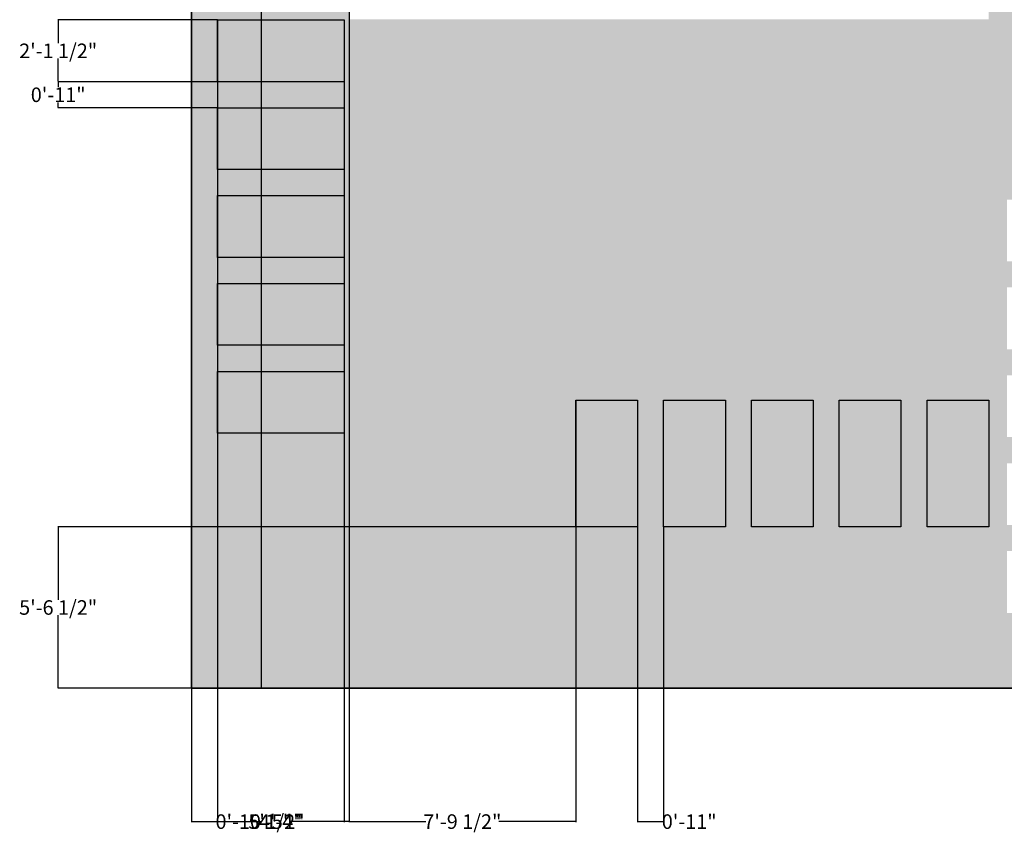
# Model space of a CAD drawing. Units: inches. Extents: x 1379 to 6665, y -118 to 1026.
# Tile 12 of 29: x 3613 to 4019, y -118 to 222. Entities that reach past the tile are written whole.
import ezdxf

# ---------------------------------------------------------------- set-up
doc = ezdxf.new("R2010")
doc.units = ezdxf.units.IN
doc.header["$MEASUREMENT"] = 0
for name, color, linetype, lineweight in [('A-ANNO-DIMS', 2, 'Continuous', 18), ('C-SITE', 3, 'Continuous', 25), ('C-SITE-PATT', 8, 'Continuous', 13)]:
    doc.layers.add(name, color=color, linetype=linetype, lineweight=lineweight)
doc.styles.get("Standard").update_dxf_attribs({"font": 'arial.ttf'})
doc.dimstyles.get("Standard").update_dxf_attribs({"dimtxt": 6, "dimasz": 0.18, "dimexe": 0.18, "dimexo": 0.0625, "dimgap": 0.09, "dimtad": 0, "dimtih": 1, "dimtoh": 1, "dimdec": 1, "dimzin": 0, "dimdsep": 46, "dimlunit": 3, "dimtxsty": 'Standard', "dimcen": 0.09, "dimclrt": 250, "dimadec": 0, "dimazin": 0, "dimtfac": 1, "dimtdec": 1, "dimtofl": 0, "dimtmove": 0, "dimatfit": 3, "dimfxl": 1, "dimtolj": 1, "dimtzin": 0, "dimarcsym": 0})

# ---------------------------------------------------------------- blocks, each defined once
blk = doc.blocks.new('*D56')
at = {"layer": 'A-ANNO-DIMS', "color": 0, "lineweight": -2, "transparency": 16777216}
for p, q in [((3715.91, 1026.26), (3712.24, 1026.26)), ((3712.42, 1026.08), (3712.42, 489.42)), ((3712.42, -53.56), (3712.42, 483.11)), ((3715.91, -53.74), (3712.24, -53.74))]:
    blk.add_line(p, q, dxfattribs=at)
at = {"layer": 'A-ANNO-DIMS', "color": 0, "transparency": 16777216}
for points in [[(3712.39, 1026.08), (3712.45, 1026.08), (3712.42, 1026.26)], [(3712.39, -53.56), (3712.45, -53.56), (3712.42, -53.74)]]:
    blk.add_solid(points, dxfattribs=at)
at = {"layer": 'Defpoints', "color": 0, "transparency": 16777216}
for p in [(3715.98, 1026.26), (3712.42, -53.74), (3715.98, -53.74)]:
    blk.add_point(p, dxfattribs=at)
at = {"layer": 'A-ANNO-DIMS', "color": 0, "transparency": 16777216, "insert": (3712.42, 486.26), "char_height": 6, "attachment_point": 5}
blk.add_mtext("\\A1;90'", dxfattribs=at)
blk = doc.blocks.new('*D168')
at = {"layer": 'A-ANNO-DIMS', "color": 0, "lineweight": -2, "transparency": 16777216}
for p, q in [((3748.48, 222.07), (3748.48, -108.92)), ((3683.47, -53.8), (3683.47, -108.92)), ((3683.65, -108.74), (3707.91, -108.74)), ((3748.3, -108.74), (3724.04, -108.74))]:
    blk.add_line(p, q, dxfattribs=at)
at = {"layer": 'A-ANNO-DIMS', "color": 0, "transparency": 16777216}
for points in [[(3683.65, -108.71), (3683.65, -108.77), (3683.47, -108.74)], [(3748.3, -108.71), (3748.3, -108.77), (3748.48, -108.74)]]:
    blk.add_solid(points, dxfattribs=at)
at = {"layer": 'Defpoints', "color": 0, "transparency": 16777216}
for p in [(3748.48, 222.13), (3683.47, -53.74), (3748.48, -108.74)]:
    blk.add_point(p, dxfattribs=at)
at = {"layer": 'A-ANNO-DIMS', "color": 250, "transparency": 16777216, "insert": (3715.98, -108.74), "char_height": 6, "attachment_point": 5}
blk.add_mtext('\\A1;5\'-5"', dxfattribs=at)
blk = doc.blocks.new('*D171')
at = {"layer": 'A-ANNO-DIMS', "color": 0, "lineweight": -2, "transparency": 16777216}
for p, q in [((3694.21, 221.86), (3694.21, -108.92)), ((3746.44, 221.86), (3746.44, -108.92)), ((3694.39, -108.74), (3712.14, -108.74)), ((3746.26, -108.74), (3728.51, -108.74))]:
    blk.add_line(p, q, dxfattribs=at)
at = {"layer": 'A-ANNO-DIMS', "color": 0, "transparency": 16777216}
for points in [[(3694.39, -108.71), (3694.39, -108.77), (3694.21, -108.74)], [(3746.26, -108.71), (3746.26, -108.77), (3746.44, -108.74)]]:
    blk.add_solid(points, dxfattribs=at)
at = {"layer": 'Defpoints', "color": 0, "transparency": 16777216}
for p in [(3694.21, 221.92), (3746.44, 221.92), (3746.44, -108.74)]:
    blk.add_point(p, dxfattribs=at)
at = {"layer": 'A-ANNO-DIMS', "color": 250, "transparency": 16777216, "insert": (3720.32, -108.74), "char_height": 6, "attachment_point": 5}
blk.add_mtext('\\A1;4\'-4"', dxfattribs=at)
blk = doc.blocks.new('*D172')
at = {"layer": 'A-ANNO-DIMS', "color": 0, "lineweight": -2, "transparency": 16777216}
for p, q in [((3694.15, 221.92), (3628.29, 221.92)), ((3628.47, 221.74), (3628.47, 212.37)), ((3628.47, 196.61), (3628.47, 205.99)), ((3694.15, 196.43), (3628.29, 196.43))]:
    blk.add_line(p, q, dxfattribs=at)
at = {"layer": 'A-ANNO-DIMS', "color": 0, "transparency": 16777216}
for points in [[(3628.44, 221.74), (3628.5, 221.74), (3628.47, 221.92)], [(3628.44, 196.61), (3628.5, 196.61), (3628.47, 196.43)]]:
    blk.add_solid(points, dxfattribs=at)
at = {"layer": 'Defpoints', "color": 0, "transparency": 16777216}
for p in [(3694.21, 221.92), (3628.47, 196.43), (3694.21, 196.43)]:
    blk.add_point(p, dxfattribs=at)
at = {"layer": 'A-ANNO-DIMS', "color": 250, "transparency": 16777216, "insert": (3628.47, 209.18), "char_height": 6, "attachment_point": 5}
blk.add_mtext('\\A1;2\'-1 1/2"', dxfattribs=at)
blk = doc.blocks.new('*D173')
at = {"layer": 'A-ANNO-DIMS', "color": 0, "lineweight": -2, "transparency": 16777216}
for p, q in [((3694.21, 51.43), (3694.21, -108.92)), ((3683.47, -53.8), (3683.47, -108.92)), ((3683.65, -108.74), (3694.03, -108.74)), ((3694.21, -108.74), (3694.39, -108.74))]:
    blk.add_line(p, q, dxfattribs=at)
at = {"layer": 'A-ANNO-DIMS', "color": 0, "transparency": 16777216}
for points in [[(3683.65, -108.71), (3683.65, -108.77), (3683.47, -108.74)], [(3694.03, -108.71), (3694.03, -108.77), (3694.21, -108.74)]]:
    blk.add_solid(points, dxfattribs=at)
at = {"layer": 'Defpoints', "color": 0, "transparency": 16777216}
for p in [(3694.21, 51.49), (3683.47, -53.74), (3694.21, -108.74)]:
    blk.add_point(p, dxfattribs=at)
at = {"layer": 'A-ANNO-DIMS', "color": 250, "transparency": 16777216, "insert": (3711.78, -108.74), "char_height": 6, "attachment_point": 5}
blk.add_mtext('\\A1;0\'-10 1/2"', dxfattribs=at)
blk = doc.blocks.new('*D174')
at = {"layer": 'A-ANNO-DIMS', "color": 0, "lineweight": -2, "transparency": 16777216}
for p, q in [((3694.15, 196.43), (3628.29, 196.43)), ((3628.47, 196.25), (3628.47, 194.21)), ((3628.47, 185.86), (3628.47, 187.91)), ((3694.15, 185.68), (3628.29, 185.68))]:
    blk.add_line(p, q, dxfattribs=at)
at = {"layer": 'A-ANNO-DIMS', "color": 0, "transparency": 16777216}
for points in [[(3628.44, 196.25), (3628.5, 196.25), (3628.47, 196.43)], [(3628.44, 185.86), (3628.5, 185.86), (3628.47, 185.68)]]:
    blk.add_solid(points, dxfattribs=at)
at = {"layer": 'Defpoints', "color": 0, "transparency": 16777216}
for p in [(3694.21, 196.43), (3628.47, 185.68), (3694.21, 185.68)]:
    blk.add_point(p, dxfattribs=at)
at = {"layer": 'A-ANNO-DIMS', "color": 250, "transparency": 16777216, "insert": (3628.47, 191.06), "char_height": 6, "attachment_point": 5}
blk.add_mtext('\\A1;0\'-11"', dxfattribs=at)
blk = doc.blocks.new('*D175')
at = {"layer": 'A-ANNO-DIMS', "color": 0, "lineweight": -2, "transparency": 16777216}
for p, q in [((3748.48, 222.07), (3748.48, -108.92)), ((3842.05, 65.05), (3842.05, -108.92)), ((3748.66, -108.74), (3780.24, -108.74)), ((3841.87, -108.74), (3810.3, -108.74))]:
    blk.add_line(p, q, dxfattribs=at)
at = {"layer": 'A-ANNO-DIMS', "color": 0, "transparency": 16777216}
for points in [[(3748.66, -108.71), (3748.66, -108.77), (3748.48, -108.74)], [(3841.87, -108.71), (3841.87, -108.77), (3842.05, -108.74)]]:
    blk.add_solid(points, dxfattribs=at)
at = {"layer": 'Defpoints', "color": 0, "transparency": 16777216}
for p in [(3748.48, 222.13), (3842.05, 65.11), (3842.05, -108.74)]:
    blk.add_point(p, dxfattribs=at)
at = {"layer": 'A-ANNO-DIMS', "color": 250, "transparency": 16777216, "insert": (3795.27, -108.74), "char_height": 6, "attachment_point": 5}
blk.add_mtext('\\A1;7\'-9 1/2"', dxfattribs=at)
blk = doc.blocks.new('*D176')
at = {"layer": 'A-ANNO-DIMS', "color": 0, "lineweight": -2, "transparency": 16777216}
for p, q in [((3841.99, 12.89), (3628.29, 12.89)), ((3628.47, 12.71), (3628.47, -17.23)), ((3628.47, -53.56), (3628.47, -23.62)), ((3683.41, -53.74), (3628.29, -53.74))]:
    blk.add_line(p, q, dxfattribs=at)
at = {"layer": 'A-ANNO-DIMS', "color": 0, "transparency": 16777216}
for points in [[(3628.44, 12.71), (3628.5, 12.71), (3628.47, 12.89)], [(3628.44, -53.56), (3628.5, -53.56), (3628.47, -53.74)]]:
    blk.add_solid(points, dxfattribs=at)
at = {"layer": 'Defpoints', "color": 0, "transparency": 16777216}
for p in [(3842.05, 12.89), (3628.47, -53.74), (3683.47, -53.74)]:
    blk.add_point(p, dxfattribs=at)
at = {"layer": 'A-ANNO-DIMS', "color": 250, "transparency": 16777216, "insert": (3628.47, -20.42), "char_height": 6, "attachment_point": 5}
blk.add_mtext('\\A1;5\'-6 1/2"', dxfattribs=at)
blk = doc.blocks.new('*D177')
at = {"layer": 'A-ANNO-DIMS', "color": 0, "lineweight": -2, "transparency": 16777216}
for p, q in [((3867.54, 12.83), (3867.54, -108.92)), ((3878.29, 12.83), (3878.29, -108.92)), ((3867.72, -108.74), (3878.11, -108.74)), ((3878.29, -108.74), (3878.47, -108.74))]:
    blk.add_line(p, q, dxfattribs=at)
at = {"layer": 'A-ANNO-DIMS', "color": 0, "transparency": 16777216}
for points in [[(3867.72, -108.71), (3867.72, -108.77), (3867.54, -108.74)], [(3878.11, -108.71), (3878.11, -108.77), (3878.29, -108.74)]]:
    blk.add_solid(points, dxfattribs=at)
at = {"layer": 'Defpoints', "color": 0, "transparency": 16777216}
for p in [(3867.54, 12.89), (3878.29, 12.89), (3878.29, -108.74)]:
    blk.add_point(p, dxfattribs=at)
at = {"layer": 'A-ANNO-DIMS', "color": 250, "transparency": 16777216, "insert": (3888.87, -108.74), "char_height": 6, "attachment_point": 5}
blk.add_mtext('\\A1;0\'-11"', dxfattribs=at)

msp = doc.modelspace()

# ---------------------------------------------------------------- hatches: boundary and pattern name
at = {"layer": 'C-SITE-PATT', "transparency": 33554590}
h = msp.add_hatch(color=256, dxfattribs=at)
h.dxf.hatch_style = 1
h.paths.add_polyline_path([(3748.48, 1026.26), (3683.47, 1026.26), (3683.47, -53.74), (3748.48, -53.74)])
h.paths.add_polyline_path([(3746.44, 221.92), (3746.44, 196.43), (3694.21, 196.43), (3694.21, 221.92)], flags=16)
h.paths.add_polyline_path([(3746.44, 185.68), (3746.44, 160.2), (3694.21, 160.2), (3694.21, 185.68)], flags=16)
h.paths.add_polyline_path([(3746.44, 149.45), (3746.44, 123.96), (3694.21, 123.96), (3694.21, 149.45)], flags=16)
h.paths.add_polyline_path([(3746.44, 113.21), (3746.44, 87.73), (3694.21, 87.73), (3694.21, 113.21)], flags=16)
h.paths.add_polyline_path([(3746.44, 76.98), (3746.44, 51.49), (3694.21, 51.49), (3694.21, 76.98)], flags=16)
h = msp.add_hatch(color=256, dxfattribs=at)
h.dxf.hatch_style = 1
h.paths.add_polyline_path([(4283.47, 1026.26), (3748.48, 1026.26), (3748.48, 721.63), (3988.48, 721.63), (4283.47, 721.57)])
h.paths.add_polyline_path([(4283.47, 721.57), (3988.48, 721.57), (3988.48, 654.13), (4246.48, 654.13), (4283.47, 654.13)])
h.paths.add_polyline_path([(4283.47, 654.13), (4246.48, 654.13), (4246.48, 470.79), (4283.47, 470.79)])
h.paths.add_polyline_path([(4084.48, 222.13), (4084.48, 243.13), (4072.48, 243.13), (4072.48, 249.13), (4070.73, 249.13), (4070.73, 273.06, 0.392996), (4048.48, 249.13, 0.392996), (4026.23, 273.06), (4026.23, 249.13), (4024.48, 249.13), (4024.48, 243.13), (4012.48, 243.13), (4012.48, 222.13), (3748.48, 222.13), (3748.48, -53.74), (4084.48, -53.74)])
h.paths.add_polyline_path([(3903.78, 65.11), (3903.78, 12.89), (3878.29, 12.89), (3878.29, 65.11)], flags=16)
h.paths.add_polyline_path([(3914.53, 65.11), (3940.01, 65.11), (3940.01, 12.89), (3914.53, 12.89)], flags=16)
h.paths.add_polyline_path([(3867.54, 65.11), (3867.54, 12.89), (3842.05, 12.89), (3842.05, 65.11)], flags=16)
h.paths.add_polyline_path([(3950.76, 65.11), (3976.25, 65.11), (3976.25, 12.89), (3950.76, 12.89)], flags=16)
h.paths.add_polyline_path([(4019.96, 147.8), (4072.19, 147.8), (4072.19, 122.32), (4019.96, 122.32)], flags=16)
h.paths.add_polyline_path([(3987, 65.11), (4012.48, 65.11), (4012.48, 12.89), (3987, 12.89)], flags=16)
h.paths.add_polyline_path([(4019.96, 111.57), (4072.19, 111.57), (4072.19, 86.08), (4019.96, 86.08)], flags=16)
h.paths.add_polyline_path([(4019.96, 75.33), (4072.19, 75.33), (4072.19, 49.85), (4019.96, 49.85)], flags=16)
h.paths.add_polyline_path([(4019.96, 39.09), (4072.19, 39.09), (4072.19, 13.61), (4019.96, 13.61)], flags=16)
h.paths.add_polyline_path([(4019.96, 2.86), (4072.19, 2.86), (4072.19, -22.63), (4019.96, -22.63)], flags=16)
h = msp.add_hatch(color=256, dxfattribs=at)
h.dxf.hatch_style = 1
h.paths.add_polyline_path([(3746.44, 221.92), (3694.21, 221.92), (3694.21, 196.43), (3746.44, 196.43)])
h.paths.add_polyline_path([(3746.44, 185.68), (3694.21, 185.68), (3694.21, 160.2), (3746.44, 160.2)])
h.paths.add_polyline_path([(3746.44, 149.45), (3694.21, 149.45), (3694.21, 123.96), (3746.44, 123.96)])
h.paths.add_polyline_path([(3746.44, 113.21), (3694.21, 113.21), (3694.21, 87.73), (3746.44, 87.73)])
h.paths.add_polyline_path([(3746.44, 76.98), (3694.21, 76.98), (3694.21, 51.49), (3746.44, 51.49)])
h = msp.add_hatch(color=256, dxfattribs=at)
h.dxf.hatch_style = 1
h.paths.add_polyline_path([(3842.05, 65.11), (3842.05, 12.89), (3867.54, 12.89), (3867.54, 65.11)])
h.paths.add_polyline_path([(3878.29, 65.11), (3878.29, 12.89), (3903.78, 12.89), (3903.78, 65.11)])
h.paths.add_polyline_path([(3914.53, 65.11), (3914.53, 12.89), (3940.01, 12.89), (3940.01, 65.11)])
h.paths.add_polyline_path([(3950.76, 65.11), (3950.76, 12.89), (3976.25, 12.89), (3976.25, 65.11)])
h.paths.add_polyline_path([(3987, 65.11), (3987, 12.89), (4012.48, 12.89), (4012.48, 65.11)])

# ---------------------------------------------------------------- linework, layer by layer
at = {"layer": 'C-SITE'}
for p, q in [((3683.47, 1026.26), (3683.47, -53.74)), ((3683.47, -53.74), (4084.48, -53.74))]:
    msp.add_line(p, q, dxfattribs=at)
for points in [[(3683.47, 1026.26), (4283.47, 1026.26), (4283.47, -53.74), (3683.47, -53.74)], [(3683.47, 1026.26), (3748.48, 1026.26), (3748.48, -53.74), (3683.47, -53.74)], [(3694.21, 221.92), (3746.44, 221.92), (3746.44, 196.43), (3694.21, 196.43)], [(3694.21, 185.68), (3746.44, 185.68), (3746.44, 160.2), (3694.21, 160.2)], [(3694.21, 149.45), (3746.44, 149.45), (3746.44, 123.96), (3694.21, 123.96)], [(3694.21, 113.21), (3746.44, 113.21), (3746.44, 87.73), (3694.21, 87.73)], [(3694.21, 76.98), (3746.44, 76.98), (3746.44, 51.49), (3694.21, 51.49)], [(3842.05, 12.89), (3842.05, 65.11), (3867.54, 65.11), (3867.54, 12.89)], [(3878.29, 12.89), (3878.29, 65.11), (3903.78, 65.11), (3903.78, 12.89)], [(3914.53, 12.89), (3914.53, 65.11), (3940.01, 65.11), (3940.01, 12.89)], [(3950.76, 12.89), (3950.76, 65.11), (3976.25, 65.11), (3976.25, 12.89)], [(3987, 12.89), (3987, 65.11), (4012.48, 65.11), (4012.48, 12.89)]]:
    msp.add_lwpolyline(points, close=True, dxfattribs=at)

# ---------------------------------------------------------------- dimensions: what is measured, and where the dimension line sits
at = {"layer": 'A-ANNO-DIMS'}
for base, p1, p2, override, picture, middle in [((3712.42, -53.74), (3715.98, 1026.26), (3715.98, -53.74), {"dimclrd": 0, "dimclre": 0, "dimclrt": 0}, '*D56', (3712.42, 486.26)), ((3628.47, 196.43), (3694.21, 221.92), (3694.21, 196.43), {"dimdec": 1, "dimlfac": 1, "dimrnd": 0, "dimzin": 1, "dimdsep": 46, "dimlunit": 4, "dimfrac": 2}, '*D172', (3628.47, 209.18)), ((3628.4696, 185.684), (3694.212, 196.4345), (3694.212, 185.684), {"dimdec": 1, "dimlfac": 1, "dimrnd": 0, "dimzin": 1, "dimdsep": 46, "dimlunit": 4, "dimfrac": 2}, '*D174', (3628.4696, 191.0592)), ((3628.47, -53.74), (3842.05, 12.89), (3683.47, -53.74), {"dimdec": 1, "dimlfac": 1, "dimrnd": 0, "dimzin": 1, "dimdsep": 46, "dimlunit": 4, "dimfrac": 2}, '*D176', (3628.47, -20.42))]:
    dim = msp.add_linear_dim(base=base, p1=p1, p2=p2, angle=90, dimstyle='Standard', override=override, dxfattribs=at)
    dim.commit()
    dim.dimension.update_dxf_attribs({"geometry": picture, "text_midpoint": middle})
for base, p1, p2, picture, middle in [((3748.48, -108.74), (3683.47, -53.74), (3748.48, 222.13), '*D168', (3715.98, -108.74)), ((3746.44, -108.74), (3694.21, 221.92), (3746.44, 221.92), '*D171', (3720.32, -108.74)), ((3842.05, -108.74), (3748.48, 222.13), (3842.05, 65.11), '*D175', (3795.27, -108.74)), ((3694.21, -108.74), (3683.47, -53.74), (3694.21, 51.49), '*D173', (3711.78, -108.74)), ((3878.2896, -108.7367), (3867.5391, 12.8891), (3878.2896, 12.8891), '*D177', (3888.8652, -108.7367))]:
    dim = msp.add_linear_dim(base=base, p1=p1, p2=p2, dimstyle='Standard', override={"dimdec": 1, "dimlfac": 1, "dimrnd": 0, "dimzin": 1, "dimdsep": 46, "dimlunit": 4, "dimfrac": 2}, dxfattribs=at)
    dim.commit()
    dim.dimension.update_dxf_attribs({"geometry": picture, "text_midpoint": middle})

doc.saveas('drawing.dxf')
